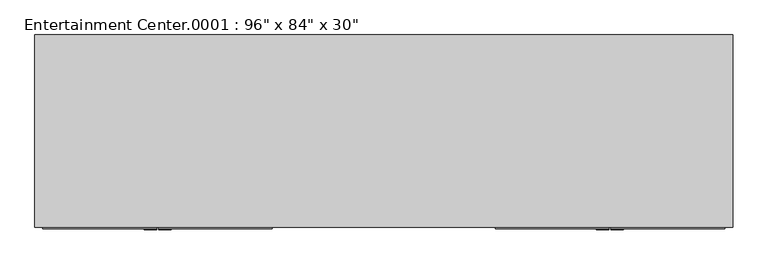
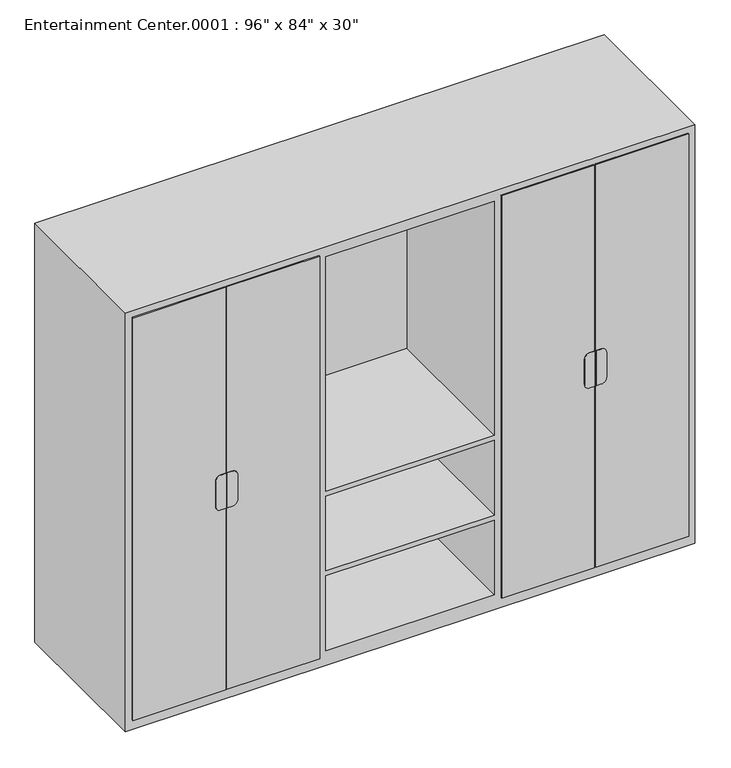
"""IFC4 building model written with IfcOpenShell, lengths in millimetres: furniture geometry."""

from ifc_helpers import new_model, si_unit, point, frame, frame_2d, origin, place, context, project, spatial, polyline, circle_curve, trimmed, segment, composite_curve, outline, extrude, faceted_brep, source, transform, mapped, element, save


def furniture_1f19b6cd(model_context):
    return source(origin(), model_context, "Body", "SolidModel", [
        extrude(outline(polyline([(-1339.85, -781.05), (-892.175, -781.05), (-892.175, -787.4), (-1339.85, -787.4), (-1339.85, -781.05)])), frame((0.0, 0.0, 50.8), z_axis=(0.0, 0.0, 1.0), x_axis=(1.0, 0.0, 0.0)), (0.0, 0.0, 1.0), 2051.05),
        extrude(outline(polyline([(-885.825, -781.05), (-438.15, -781.05), (-438.15, -787.4), (-885.825, -787.4), (-885.825, -781.05)])), frame((0.0, 0.0, 50.8), z_axis=(0.0, 0.0, 1.0), x_axis=(1.0, 0.0, 0.0)), (0.0, 0.0, 1.0), 2051.05),
        extrude(outline(polyline([(892.175, -781.05), (1339.85, -781.05), (1339.85, -787.4), (892.175, -787.4), (892.175, -781.05)])), frame((0.0, 0.0, 50.8), z_axis=(0.0, 0.0, 1.0), x_axis=(1.0, 0.0, 0.0)), (0.0, 0.0, 1.0), 2051.05),
        extrude(outline(polyline([(438.15, -781.05), (885.825, -781.05), (885.825, -787.4), (438.15, -787.4), (438.15, -781.05)])), frame((0.0, 0.0, 50.8), z_axis=(0.0, 0.0, 1.0), x_axis=(1.0, 0.0, 0.0)), (0.0, 0.0, 1.0), 2051.05),
        extrude(outline(composite_curve([segment(polyline([(1155.7, -861.5986452), (1155.7, -885.825), (977.9, -885.825), (977.9, -861.5986452)]), True, "CONTINUOUS"), segment(trimmed(circle_curve(frame_2d((1003.3, -861.5986452)), 25.4), [point((977.9, -861.5986452))], [point((1003.3, -836.1986452))], False, "CARTESIAN"), True, "CONTINUOUS"), segment(polyline([(1003.3, -836.1986452), (1130.3, -836.1986452)]), True, "CONTINUOUS"), segment(trimmed(circle_curve(frame_2d((1130.3, -861.5986452)), 25.4), [point((1130.3, -836.1986452))], [point((1155.7, -861.5986452))], False, "CARTESIAN"), True, "CONTINUOUS")], self_intersect=False)), frame((0.0, -790.575, 0.0), z_axis=(0.0, 1.0, 0.0), x_axis=(0.0, 0.0, 1.0)), (0.0, 0.0, 1.0), 3.175),
        extrude(outline(composite_curve([segment(trimmed(circle_curve(frame_2d((1130.3, -916.78125)), 25.4), [point((1155.7, -916.78125))], [point((1130.3, -942.18125))], False, "CARTESIAN"), True, "CONTINUOUS"), segment(polyline([(1130.3, -942.18125), (1003.3, -942.18125)]), True, "CONTINUOUS"), segment(trimmed(circle_curve(frame_2d((1003.3, -916.78125)), 25.4), [point((1003.3, -942.18125))], [point((977.9, -916.78125))], False, "CARTESIAN"), True, "CONTINUOUS"), segment(polyline([(977.9, -916.78125), (977.9, -892.175), (1155.7, -892.175), (1155.7, -916.78125)]), True, "CONTINUOUS")], self_intersect=False)), frame((0.0, -790.575, 0.0), z_axis=(0.0, 1.0, 0.0), x_axis=(0.0, 0.0, 1.0)), (0.0, 0.0, 1.0), 3.175),
        extrude(outline(composite_curve([segment(trimmed(circle_curve(frame_2d((1130.3, 861.5986452)), 25.4), [point((1155.7, 861.5986452))], [point((1130.3, 836.1986452))], False, "CARTESIAN"), True, "CONTINUOUS"), segment(polyline([(1130.3, 836.1986452), (1003.3, 836.1986452)]), True, "CONTINUOUS"), segment(trimmed(circle_curve(frame_2d((1003.3, 861.5986452)), 25.4), [point((1003.3, 836.1986452))], [point((977.9, 861.5986452))], False, "CARTESIAN"), True, "CONTINUOUS"), segment(polyline([(977.9, 861.5986452), (977.9, 885.825), (1155.7, 885.825), (1155.7, 861.5986452)]), True, "CONTINUOUS")], self_intersect=False)), frame((0.0, -790.575, 0.0), z_axis=(0.0, 1.0, 0.0), x_axis=(0.0, 0.0, 1.0)), (0.0, 0.0, 1.0), 3.175),
        extrude(outline(composite_curve([segment(polyline([(1155.7, 916.78125), (1155.7, 892.175), (977.9, 892.175), (977.9, 916.78125)]), True, "CONTINUOUS"), segment(trimmed(circle_curve(frame_2d((1003.3, 916.78125)), 25.4), [point((977.9, 916.78125))], [point((1003.3, 942.18125))], False, "CARTESIAN"), True, "CONTINUOUS"), segment(polyline([(1003.3, 942.18125), (1130.3, 942.18125)]), True, "CONTINUOUS"), segment(trimmed(circle_curve(frame_2d((1130.3, 916.78125)), 25.4), [point((1130.3, 942.18125))], [point((1155.7, 916.78125))], False, "CARTESIAN"), True, "CONTINUOUS")], self_intersect=False)), frame((0.0, -790.575, 0.0), z_axis=(0.0, 1.0, 0.0), x_axis=(0.0, 0.0, 1.0)), (0.0, 0.0, 1.0), 3.175),
        faceted_brep([(1371.6, -781.05, 0.0), (1371.6, -781.05, 2133.6), (-1371.6, -781.05, 2133.6), (-1371.6, -781.05, 0.0), (-457.2, -781.05, 2082.8), (-457.2, -781.05, 1612.9), (-1320.8, -781.05, 1612.9), (-1320.8, -781.05, 2082.8), (-457.2, -781.05, 76.2), (-1320.8, -781.05, 76.2), (-1320.8, -781.05, 520.7), (-457.2, -781.05, 520.7), (1320.8, -781.05, 1612.9), (457.2, -781.05, 1612.9), (457.2, -781.05, 2082.8), (1320.8, -781.05, 2082.8), (-406.4, -781.05, 889.0), (-406.4, -781.05, 2082.8), (406.4, -781.05, 2082.8), (406.4, -781.05, 889.0), (406.4, -781.05, 76.2), (-406.4, -781.05, 76.2), (-406.4, -781.05, 457.2), (406.4, -781.05, 457.2), (1320.8, -781.05, 76.2), (457.2, -781.05, 76.2), (457.2, -781.05, 520.7), (1320.8, -781.05, 520.7), (-1320.8, -781.05, 546.1), (-1320.8, -781.05, 1054.1), (-457.2, -781.05, 1054.1), (-457.2, -781.05, 546.1), (-457.2, -781.05, 1587.5), (-457.2, -781.05, 1079.5), (-1320.8, -781.05, 1079.5), (-1320.8, -781.05, 1587.5), (457.2, -781.05, 1587.5), (1320.8, -781.05, 1587.5), (1320.8, -781.05, 1079.5), (457.2, -781.05, 1079.5), (457.2, -781.05, 1054.1), (1320.8, -781.05, 1054.1), (1320.8, -781.05, 546.1), (457.2, -781.05, 546.1), (406.4, -781.05, 482.6), (-406.4, -781.05, 482.6), (-406.4, -781.05, 863.6), (406.4, -781.05, 863.6), (1371.6, -25.4, 0.0), (-1371.6, -25.4, 0.0), (-1371.6, -25.4, 2133.6), (1371.6, -25.4, 2133.6), (-457.2, -50.8, 2082.8), (-457.2, -50.8, 1612.9), (-1320.8, -50.8, 1612.9), (-1320.8, -50.8, 2082.8), (-457.2, -50.8, 76.2), (-1320.8, -50.8, 76.2), (-1320.8, -50.8, 520.7), (-457.2, -50.8, 520.7), (1320.8, -50.8, 1612.9), (457.2, -50.8, 1612.9), (457.2, -50.8, 2082.8), (1320.8, -50.8, 2082.8), (-406.4, -50.8, 889.0), (-406.4, -50.8, 2082.8), (406.4, -50.8, 2082.8), (406.4, -50.8, 889.0), (406.4, -50.8, 76.2), (-406.4, -50.8, 76.2), (-406.4, -50.8, 457.2), (406.4, -50.8, 457.2), (1320.8, -50.8, 76.2), (457.2, -50.8, 76.2), (457.2, -50.8, 520.7), (1320.8, -50.8, 520.7), (-1320.8, -50.8, 546.1), (-1320.8, -50.8, 1054.1), (-457.2, -50.8, 1054.1), (-457.2, -50.8, 546.1), (-457.2, -50.8, 1587.5), (-457.2, -50.8, 1079.5), (-1320.8, -50.8, 1079.5), (-1320.8, -50.8, 1587.5), (457.2, -50.8, 1587.5), (1320.8, -50.8, 1587.5), (1320.8, -50.8, 1079.5), (457.2, -50.8, 1079.5), (457.2, -50.8, 1054.1), (1320.8, -50.8, 1054.1), (1320.8, -50.8, 546.1), (457.2, -50.8, 546.1), (406.4, -50.8, 482.6), (-406.4, -50.8, 482.6), (-406.4, -50.8, 863.6), (406.4, -50.8, 863.6)], [[[0, 1, 2, 3], [4, 5, 6, 7], [8, 9, 10, 11], [12, 13, 14, 15], [16, 17, 18, 19], [20, 21, 22, 23], [24, 25, 26, 27], [28, 29, 30, 31], [32, 33, 34, 35], [36, 37, 38, 39], [40, 41, 42, 43], [44, 45, 46, 47]], [[48, 49, 50, 51]], [[1, 0, 48, 51]], [[2, 1, 51, 50]], [[3, 2, 50, 49]], [[0, 3, 49, 48]], [[5, 4, 52, 53]], [[6, 5, 53, 54]], [[7, 6, 54, 55]], [[4, 7, 55, 52]], [[9, 8, 56, 57]], [[10, 9, 57, 58]], [[11, 10, 58, 59]], [[8, 11, 59, 56]], [[13, 12, 60, 61]], [[14, 13, 61, 62]], [[15, 14, 62, 63]], [[12, 15, 63, 60]], [[17, 16, 64, 65]], [[18, 17, 65, 66]], [[19, 18, 66, 67]], [[16, 19, 67, 64]], [[21, 20, 68, 69]], [[22, 21, 69, 70]], [[23, 22, 70, 71]], [[20, 23, 71, 68]], [[25, 24, 72, 73]], [[26, 25, 73, 74]], [[27, 26, 74, 75]], [[24, 27, 75, 72]], [[29, 28, 76, 77]], [[30, 29, 77, 78]], [[31, 30, 78, 79]], [[28, 31, 79, 76]], [[33, 32, 80, 81]], [[34, 33, 81, 82]], [[35, 34, 82, 83]], [[32, 35, 83, 80]], [[37, 36, 84, 85]], [[38, 37, 85, 86]], [[39, 38, 86, 87]], [[36, 39, 87, 84]], [[41, 40, 88, 89]], [[42, 41, 89, 90]], [[43, 42, 90, 91]], [[40, 43, 91, 88]], [[45, 44, 92, 93]], [[46, 45, 93, 94]], [[47, 46, 94, 95]], [[44, 47, 95, 92]], [[53, 52, 55, 54]], [[57, 56, 59, 58]], [[61, 60, 63, 62]], [[65, 64, 67, 66]], [[69, 68, 71, 70]], [[73, 72, 75, 74]], [[77, 76, 79, 78]], [[81, 80, 83, 82]], [[85, 84, 87, 86]], [[89, 88, 91, 90]], [[93, 92, 95, 94]]]),
    ])


if __name__ == "__main__":
    model = new_model("IFC4")
    model_context = context("Model", 3, world=origin())
    ifc_project = project(units=[si_unit("LENGTHUNIT", "METRE", prefix="MILLI")], contexts=[model_context])
    site = spatial("IfcSite", under=ifc_project)
    building = spatial("IfcBuilding", under=site)
    placement = place(None, origin())
    furniture_shape = furniture_1f19b6cd(model_context)
    element("IfcFurniture", 1, ObjectType="Entertainment Center.0001 : 96\" x 84\" x 30\"", at=placement, inside=building, context=model_context, shape_type="MappedRepresentation", body=[
        mapped(furniture_shape, transform((0.0, 0.0, 0.0), x_axis=(1.0, 0.0, 0.0), y_axis=(0.0, 1.0, 0.0), z_axis=(0.0, 0.0, 1.0))),
    ])
    save(model, "model.ifc")

# Revit data of these elements
# Type "Entertainment Center.0001 : 96\" x 84\" x 30\""
#   Assembly Code = "E2020200"
#   Center Width = 2' - 8"
#   Depth = 2' - 6"
#   Height = 7' - 0"
#   Width = 9' - 0"
#   Material = Laminate, Ivory, Matte
#   Default Elevation = 0
# Element 1 (IfcFurniture, "Entertainment Center.0001 : 96\" x 84\" x 30\"")
#   Materials on its faces: "Laminate, Ivory, Matte", "Steel, Chrome Plated", "Glass - Clear, Grey"
# Materials
#   "Laminate, Ivory, Matte": class "Plastic", colour RGB 247 247 239, transparency 0, Description = "Plastic Laminate - Ivory, Matte", Cost = 0
#   "Steel, Chrome Plated": class "Metal", colour RGB 17 17 17, transparency 0, Description = "Chromiuim plated steel", Cost = 0
#   "Glass - Clear, Grey": class "Glass", colour RGB 252 255 255, transparency 0.64
